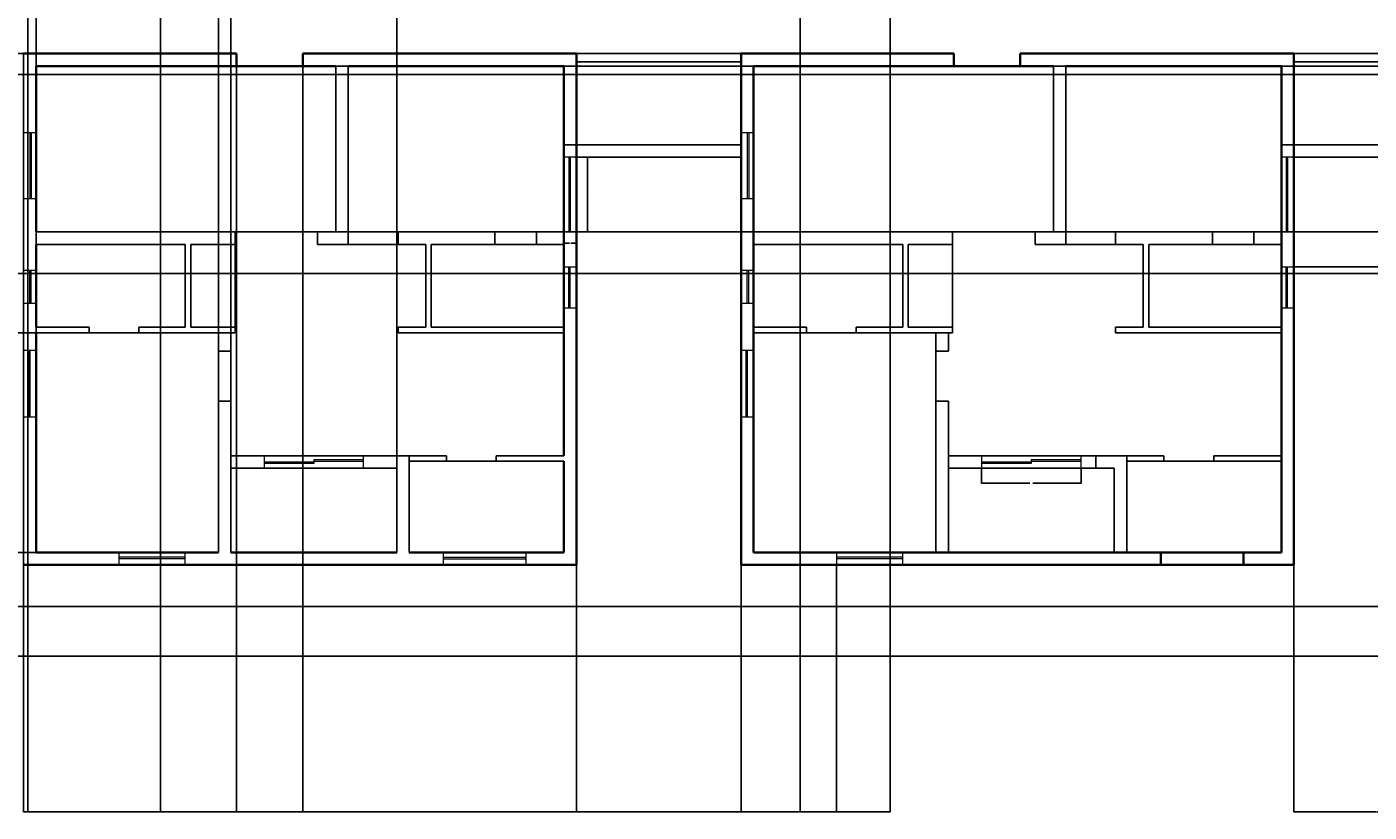
# Model space of a CAD drawing. Units: inches. Extents: x 2029 to 8798, y 1998 to 6373.
# Tile 4 of 11: x 2855 to 3826, y 4031 to 4599. Entities that reach past the tile are written whole.
import ezdxf

# ---------------------------------------------------------------- set-up
doc = ezdxf.new("R2010")
doc.units = ezdxf.units.IN
for name, color, linetype, lineweight in [('A-ANNO-DIMS', 2, 'Continuous', 18), ('A-GLAZ', 4, 'Continuous', 18), ('A-WALL-CIRC', 7, 'Continuous', 25), ('A-WALL-EXTR', 7, 'Continuous', 35), ('A-WALL-INTR', 7, 'Continuous', 25)]:
    doc.layers.add(name, color=color, linetype=linetype, lineweight=lineweight)
doc.styles.get("Standard").update_dxf_attribs({"font": 'arial.ttf'})
doc.dimstyles.get("Standard").update_dxf_attribs({"dimtxt": 0.18, "dimasz": 0.18, "dimexe": 0.18, "dimexo": 0.0625, "dimgap": 0.09, "dimtad": 0, "dimtih": 1, "dimtoh": 1, "dimdec": 4, "dimzin": 0, "dimdsep": 46, "dimtxsty": 'Standard', "dimcen": 0.09, "dimadec": 0, "dimazin": 0, "dimtfac": 1, "dimtdec": 4, "dimtofl": 0, "dimtmove": 0, "dimatfit": 3, "dimfxl": 1, "dimtolj": 1, "dimtzin": 0, "dimarcsym": 0})

# ---------------------------------------------------------------- blocks, each defined once
blk = doc.blocks.new('WIN-60')
for p, q in [((0, 0), (0, 9)), ((0, 4.5), (60, 4.5)), ((0, 3.5), (60, 3.5)), ((60, 9), (60, 0))]:
    blk.add_line(p, q)
blk = doc.blocks.new('WIN-48')
for p, q in [((0, 48), (9, 48)), ((4.5, 48), (4.5, 0)), ((5.5, 48), (5.5, 0)), ((9, 0), (0, 0))]:
    blk.add_line(p, q)
blk = doc.blocks.new('WIN-30')
for p, q in [((0, 0), (0, 9)), ((0, 5.5), (30, 5.5)), ((0, 4.5), (30, 4.5)), ((30, 9), (30, 0))]:
    blk.add_line(p, q)
blk = doc.blocks.new('WIN-24')
for p, q in [((0, 0), (0, 9)), ((0, 4.5), (24, 4.5)), ((0, 3.5), (24, 3.5)), ((24, 9), (24, 0))]:
    blk.add_line(p, q)
blk = doc.blocks.new('GLAZ-SLIDER-72-H')
for p, q in [((0, 9), (0, 0)), ((0, 4.5), (36, 4.5)), ((36, 3.5), (0, 3.5)), ((72, 6), (36, 6)), ((36, 6), (36, 5)), ((36, 5), (72, 5)), ((36, 4.5), (36, 3.5)), ((36, 4.5), (36, 4.5)), ((72, 0), (72, 9)), ((72, 5), (72, 6))]:
    blk.add_line(p, q)
blk = doc.blocks.new('WIN-54')
for p, q in [((9, 54), (0, 54)), ((3.5, 54), (3.5, 0)), ((4.5, 54), (4.5, 0)), ((0, 0), (9, 0))]:
    blk.add_line(p, q)
blk = doc.blocks.new('*D29')
at = {"layer": 'A-ANNO-DIMS', "color": 0, "lineweight": -2, "transparency": 16777216}
for p, q in [((3545.77, 4279.93), (3545.77, 4269.01)), ((3617.77, 4279.93), (3617.77, 4269.01)), ((3545.95, 4269.19), (3580.75, 4269.19)), ((3617.59, 4269.19), (3582.78, 4269.19))]:
    blk.add_line(p, q, dxfattribs=at)
at = {"layer": 'A-ANNO-DIMS', "color": 0, "transparency": 16777216}
for points in [[(3545.95, 4269.22), (3545.95, 4269.16), (3545.77, 4269.19)], [(3617.59, 4269.22), (3617.59, 4269.16), (3617.77, 4269.19)]]:
    blk.add_solid(points, dxfattribs=at)
at = {"layer": 'Defpoints', "color": 0, "transparency": 16777216}
for p in [(3545.77, 4279.99), (3617.77, 4279.99), (3617.77, 4269.19)]:
    blk.add_point(p, dxfattribs=at)
at = {"layer": 'A-ANNO-DIMS', "color": 0, "transparency": 16777216, "insert": (3581.77, 4269.19), "char_height": 0.18, "attachment_point": 5}
blk.add_mtext('\\A1;SLIDER 72 TYP.', dxfattribs=at)
blk = doc.blocks.new('*D30')
at = {"layer": 'A-ANNO-DIMS', "color": 0, "lineweight": -2, "transparency": 16777216}
for p, q in [((3617.83, 4288.99), (3628.75, 4288.99)), ((3628.57, 4288.81), (3628.57, 4284.67)), ((3628.57, 4280.17), (3628.57, 4284.31)), ((3617.83, 4279.99), (3628.75, 4279.99))]:
    blk.add_line(p, q, dxfattribs=at)
at = {"layer": 'A-ANNO-DIMS', "color": 0, "transparency": 16777216}
for points in [[(3628.54, 4288.81), (3628.6, 4288.81), (3628.57, 4288.99)], [(3628.54, 4280.17), (3628.6, 4280.17), (3628.57, 4279.99)]]:
    blk.add_solid(points, dxfattribs=at)
at = {"layer": 'Defpoints', "color": 0, "transparency": 16777216}
for p in [(3617.77, 4288.99), (3628.57, 4288.99), (3617.77, 4279.99)]:
    blk.add_point(p, dxfattribs=at)
at = {"layer": 'A-ANNO-DIMS', "color": 0, "transparency": 16777216, "insert": (3628.57, 4284.49), "char_height": 0.18, "attachment_point": 5}
blk.add_mtext('\\A1;9 TYP.', dxfattribs=at)
blk = doc.blocks.new('*D31')
at = {"layer": 'A-ANNO-DIMS', "color": 0, "lineweight": -2, "transparency": 16777216}
for p, q in [((3252.6, 4504.99), (3260.82, 4504.99)), ((3260.64, 4504.81), (3260.64, 4478.17)), ((3260.64, 4451.17), (3260.64, 4477.81)), ((3252.6, 4450.99), (3260.82, 4450.99))]:
    blk.add_line(p, q, dxfattribs=at)
at = {"layer": 'A-ANNO-DIMS', "color": 0, "transparency": 16777216}
for points in [[(3260.61, 4504.81), (3260.67, 4504.81), (3260.64, 4504.99)], [(3260.61, 4451.17), (3260.67, 4451.17), (3260.64, 4450.99)]]:
    blk.add_solid(points, dxfattribs=at)
at = {"layer": 'Defpoints', "color": 0, "transparency": 16777216}
for p in [(3252.54, 4504.99), (3260.64, 4504.99), (3252.54, 4450.99)]:
    blk.add_point(p, dxfattribs=at)
at = {"layer": 'A-ANNO-DIMS', "color": 0, "transparency": 16777216, "insert": (3260.64, 4477.99), "char_height": 0.18, "attachment_point": 5}
blk.add_mtext('\\A1;WINDOW 54 TYP.', dxfattribs=at)
blk = doc.blocks.new('*D32')
at = {"layer": 'A-ANNO-DIMS', "color": 0, "lineweight": -2, "transparency": 16777216}
for p, q in [((3243.54, 4450.93), (3243.54, 4442.71)), ((3252.54, 4450.93), (3252.54, 4442.71)), ((3243.72, 4442.89), (3247.58, 4442.89)), ((3252.36, 4442.89), (3248.5, 4442.89))]:
    blk.add_line(p, q, dxfattribs=at)
at = {"layer": 'A-ANNO-DIMS', "color": 0, "transparency": 16777216}
for points in [[(3243.72, 4442.92), (3243.72, 4442.86), (3243.54, 4442.89)], [(3252.36, 4442.92), (3252.36, 4442.86), (3252.54, 4442.89)]]:
    blk.add_solid(points, dxfattribs=at)
at = {"layer": 'Defpoints', "color": 0, "transparency": 16777216}
for p in [(3243.54, 4450.99), (3252.54, 4450.99), (3252.54, 4442.89)]:
    blk.add_point(p, dxfattribs=at)
at = {"layer": 'A-ANNO-DIMS', "color": 0, "transparency": 16777216, "insert": (3248.04, 4442.89), "char_height": 0.18, "attachment_point": 5}
blk.add_mtext('\\A1;9 TYP.', dxfattribs=at)
blk = doc.blocks.new('*D39')
at = {"layer": 'A-ANNO-DIMS', "color": 0, "lineweight": -2, "transparency": 16777216}
for p, q in [((2852.54, 4209.93), (2852.54, 4031.06)), ((3252.54, 4209.93), (3252.54, 4031.06)), ((2852.72, 4031.24), (3052.25, 4031.24)), ((3252.36, 4031.24), (3052.83, 4031.24))]:
    blk.add_line(p, q, dxfattribs=at)
at = {"layer": 'A-ANNO-DIMS', "color": 0, "transparency": 16777216}
for points in [[(2852.72, 4031.27), (2852.72, 4031.21), (2852.54, 4031.24)], [(3252.36, 4031.27), (3252.36, 4031.21), (3252.54, 4031.24)]]:
    blk.add_solid(points, dxfattribs=at)
at = {"layer": 'Defpoints', "color": 0, "transparency": 16777216}
for p in [(2852.54, 4209.99), (3252.54, 4209.99), (3252.54, 4031.24)]:
    blk.add_point(p, dxfattribs=at)
at = {"layer": 'A-ANNO-DIMS', "color": 0, "transparency": 16777216, "insert": (3052.54, 4031.24), "char_height": 0.18, "attachment_point": 5}
blk.add_mtext('\\A1;400', dxfattribs=at)
blk = doc.blocks.new('*D40')
at = {"layer": 'A-ANNO-DIMS', "color": 0, "lineweight": -2, "transparency": 16777216}
for p, q in [((3252.54, 4209.93), (3252.54, 4031.06)), ((3371.77, 4209.93), (3371.77, 4031.06)), ((3252.72, 4031.24), (3311.7, 4031.24)), ((3371.59, 4031.24), (3312.61, 4031.24))]:
    blk.add_line(p, q, dxfattribs=at)
at = {"layer": 'A-ANNO-DIMS', "color": 0, "transparency": 16777216}
for points in [[(3252.72, 4031.27), (3252.72, 4031.21), (3252.54, 4031.24)], [(3371.59, 4031.27), (3371.59, 4031.21), (3371.77, 4031.24)]]:
    blk.add_solid(points, dxfattribs=at)
at = {"layer": 'Defpoints', "color": 0, "transparency": 16777216}
for p in [(3252.54, 4209.99), (3371.77, 4209.99), (3371.77, 4031.24)]:
    blk.add_point(p, dxfattribs=at)
at = {"layer": 'A-ANNO-DIMS', "color": 0, "transparency": 16777216, "insert": (3312.15, 4031.24), "char_height": 0.18, "attachment_point": 5}
blk.add_mtext('\\A1;119.23', dxfattribs=at)
blk = doc.blocks.new('*D41')
at = {"layer": 'A-ANNO-DIMS', "color": 0, "lineweight": -2, "transparency": 16777216}
for p, q in [((3771.77, 4209.93), (3771.77, 4031.06)), ((3890.77, 4179.93), (3890.77, 4031.06)), ((3771.95, 4031.24), (3830.99, 4031.24)), ((3890.59, 4031.24), (3831.55, 4031.24))]:
    blk.add_line(p, q, dxfattribs=at)
at = {"layer": 'A-ANNO-DIMS', "color": 0, "transparency": 16777216}
for points in [[(3771.95, 4031.27), (3771.95, 4031.21), (3771.77, 4031.24)], [(3890.59, 4031.27), (3890.59, 4031.21), (3890.77, 4031.24)]]:
    blk.add_solid(points, dxfattribs=at)
at = {"layer": 'Defpoints', "color": 0, "transparency": 16777216}
for p in [(3771.77, 4209.99), (3890.77, 4179.99), (3890.77, 4031.24)]:
    blk.add_point(p, dxfattribs=at)
at = {"layer": 'A-ANNO-DIMS', "color": 0, "transparency": 16777216, "insert": (3831.27, 4031.24), "char_height": 0.18, "attachment_point": 5}
blk.add_mtext('\\A1;119', dxfattribs=at)
blk = doc.blocks.new('*D50')
at = {"layer": 'A-ANNO-DIMS', "color": 0, "lineweight": -2, "transparency": 16777216}
for p, q in [((2852.54, 4579.93), (2852.54, 4031.06)), ((3006.54, 4579.93), (3006.54, 4031.06)), ((2852.72, 4031.24), (2929.26, 4031.24)), ((3006.36, 4031.24), (2929.82, 4031.24))]:
    blk.add_line(p, q, dxfattribs=at)
at = {"layer": 'A-ANNO-DIMS', "color": 0, "transparency": 16777216}
for points in [[(2852.72, 4031.27), (2852.72, 4031.21), (2852.54, 4031.24)], [(3006.36, 4031.27), (3006.36, 4031.21), (3006.54, 4031.24)]]:
    blk.add_solid(points, dxfattribs=at)
at = {"layer": 'Defpoints', "color": 0, "transparency": 16777216}
for p in [(2852.54, 4579.99), (3006.54, 4579.99), (3006.54, 4031.24)]:
    blk.add_point(p, dxfattribs=at)
at = {"layer": 'A-ANNO-DIMS', "color": 0, "transparency": 16777216, "insert": (2929.54, 4031.24), "char_height": 0.18, "attachment_point": 5}
blk.add_mtext('\\A1;154', dxfattribs=at)
blk = doc.blocks.new('*D51')
at = {"layer": 'A-ANNO-DIMS', "color": 0, "lineweight": -2, "transparency": 16777216}
for p, q in [((3006.54, 4579.93), (3006.54, 4031.06)), ((3054.54, 4579.93), (3054.54, 4031.06)), ((3006.72, 4031.24), (3030.32, 4031.24)), ((3054.36, 4031.24), (3030.76, 4031.24))]:
    blk.add_line(p, q, dxfattribs=at)
at = {"layer": 'A-ANNO-DIMS', "color": 0, "transparency": 16777216}
for points in [[(3006.72, 4031.27), (3006.72, 4031.21), (3006.54, 4031.24)], [(3054.36, 4031.27), (3054.36, 4031.21), (3054.54, 4031.24)]]:
    blk.add_solid(points, dxfattribs=at)
at = {"layer": 'Defpoints', "color": 0, "transparency": 16777216}
for p in [(3006.54, 4579.99), (3054.54, 4579.99), (3054.54, 4031.24)]:
    blk.add_point(p, dxfattribs=at)
at = {"layer": 'A-ANNO-DIMS', "color": 0, "transparency": 16777216, "insert": (3030.54, 4031.24), "char_height": 0.18, "attachment_point": 5}
blk.add_mtext('\\A1;48', dxfattribs=at)
blk = doc.blocks.new('*D52')
at = {"layer": 'A-ANNO-DIMS', "color": 0, "lineweight": -2, "transparency": 16777216}
for p, q in [((2861.6, 4570.99), (4503.7, 4570.99)), ((4503.52, 4570.81), (4503.52, 4511.17)), ((4503.52, 4451.17), (4503.52, 4510.81)), ((2861.6, 4450.99), (4503.7, 4450.99))]:
    blk.add_line(p, q, dxfattribs=at)
at = {"layer": 'A-ANNO-DIMS', "color": 0, "transparency": 16777216}
for points in [[(4503.49, 4570.81), (4503.55, 4570.81), (4503.52, 4570.99)], [(4503.49, 4451.17), (4503.55, 4451.17), (4503.52, 4450.99)]]:
    blk.add_solid(points, dxfattribs=at)
at = {"layer": 'Defpoints', "color": 0, "transparency": 16777216}
for p in [(2861.54, 4570.99), (4503.52, 4570.99), (2861.54, 4450.99)]:
    blk.add_point(p, dxfattribs=at)
at = {"layer": 'A-ANNO-DIMS', "color": 0, "transparency": 16777216, "insert": (4503.52, 4510.99), "char_height": 0.18, "attachment_point": 5}
blk.add_mtext('\\A1;120', dxfattribs=at)
blk = doc.blocks.new('*D53')
at = {"layer": 'A-ANNO-DIMS', "color": 0, "lineweight": -2, "transparency": 16777216}
for p, q in [((2861.48, 4377.99), (2029.61, 4377.99)), ((2029.79, 4377.81), (2029.79, 4298.67)), ((2029.79, 4219.17), (2029.79, 4298.31)), ((2861.48, 4218.99), (2029.61, 4218.99))]:
    blk.add_line(p, q, dxfattribs=at)
at = {"layer": 'A-ANNO-DIMS', "color": 0, "transparency": 16777216}
for points in [[(2029.76, 4377.81), (2029.82, 4377.81), (2029.79, 4377.99)], [(2029.76, 4219.17), (2029.82, 4219.17), (2029.79, 4218.99)]]:
    blk.add_solid(points, dxfattribs=at)
at = {"layer": 'Defpoints', "color": 0, "transparency": 16777216}
for p in [(2861.54, 4377.99), (2029.79, 4218.99), (2861.54, 4218.99)]:
    blk.add_point(p, dxfattribs=at)
at = {"layer": 'A-ANNO-DIMS', "color": 0, "transparency": 16777216, "insert": (2029.79, 4298.49), "char_height": 0.18, "attachment_point": 5}
blk.add_mtext('\\A1;159', dxfattribs=at)
blk = doc.blocks.new('*D54')
at = {"layer": 'A-ANNO-DIMS', "color": 0, "lineweight": -2, "transparency": 16777216}
for p, q in [((2861.54, 4219.05), (2861.54, 6372.54)), ((2861.72, 6372.36), (2927.26, 6372.36)), ((2993.36, 6372.36), (2927.82, 6372.36)), ((2993.54, 4219.05), (2993.54, 6372.54))]:
    blk.add_line(p, q, dxfattribs=at)
at = {"layer": 'A-ANNO-DIMS', "color": 0, "transparency": 16777216}
for points in [[(2861.72, 6372.39), (2861.72, 6372.33), (2861.54, 6372.36)], [(2993.36, 6372.39), (2993.36, 6372.33), (2993.54, 6372.36)]]:
    blk.add_solid(points, dxfattribs=at)
at = {"layer": 'Defpoints', "color": 0, "transparency": 16777216}
for p in [(2993.54, 6372.36), (2861.54, 4218.99), (2993.54, 4218.99)]:
    blk.add_point(p, dxfattribs=at)
at = {"layer": 'A-ANNO-DIMS', "color": 0, "transparency": 16777216, "insert": (2927.54, 6372.36), "char_height": 0.18, "attachment_point": 5}
blk.add_mtext('\\A1;132', dxfattribs=at)
blk = doc.blocks.new('*D55')
at = {"layer": 'A-ANNO-DIMS', "color": 0, "lineweight": -2, "transparency": 16777216}
for p, q in [((3002.54, 4219.05), (3002.54, 6372.54)), ((3002.72, 6372.36), (3062.26, 6372.36)), ((3122.36, 6372.36), (3062.82, 6372.36)), ((3122.54, 4219.05), (3122.54, 6372.54))]:
    blk.add_line(p, q, dxfattribs=at)
at = {"layer": 'A-ANNO-DIMS', "color": 0, "transparency": 16777216}
for points in [[(3002.72, 6372.39), (3002.72, 6372.33), (3002.54, 6372.36)], [(3122.36, 6372.39), (3122.36, 6372.33), (3122.54, 6372.36)]]:
    blk.add_solid(points, dxfattribs=at)
at = {"layer": 'Defpoints', "color": 0, "transparency": 16777216}
for p in [(3122.54, 6372.36), (3002.54, 4218.99), (3122.54, 4218.99)]:
    blk.add_point(p, dxfattribs=at)
at = {"layer": 'A-ANNO-DIMS', "color": 0, "transparency": 16777216, "insert": (3062.54, 6372.36), "char_height": 0.18, "attachment_point": 5}
blk.add_mtext('\\A1;120', dxfattribs=at)
blk = doc.blocks.new('*D56')
at = {"layer": 'A-ANNO-DIMS', "color": 0, "lineweight": -2, "transparency": 16777216}
for p, q in [((3371.77, 4209.93), (3371.77, 4031.06)), ((3440.77, 4209.93), (3440.77, 4031.06)), ((3371.95, 4031.24), (3406.05, 4031.24)), ((3440.59, 4031.24), (3406.49, 4031.24))]:
    blk.add_line(p, q, dxfattribs=at)
at = {"layer": 'A-ANNO-DIMS', "color": 0, "transparency": 16777216}
for points in [[(3371.95, 4031.27), (3371.95, 4031.21), (3371.77, 4031.24)], [(3440.59, 4031.27), (3440.59, 4031.21), (3440.77, 4031.24)]]:
    blk.add_solid(points, dxfattribs=at)
at = {"layer": 'Defpoints', "color": 0, "transparency": 16777216}
for p in [(3371.77, 4209.99), (3440.77, 4209.99), (3440.77, 4031.24)]:
    blk.add_point(p, dxfattribs=at)
at = {"layer": 'A-ANNO-DIMS', "color": 0, "transparency": 16777216, "insert": (3406.27, 4031.24), "char_height": 0.18, "attachment_point": 5}
blk.add_mtext('\\A1;69', dxfattribs=at)
blk = doc.blocks.new('*D57')
at = {"layer": 'A-ANNO-DIMS', "color": 0, "lineweight": -2, "transparency": 16777216}
for p, q in [((3771.83, 4579.99), (4503.7, 4579.99)), ((4503.52, 4579.81), (4503.52, 4542.67)), ((4503.52, 4505.17), (4503.52, 4542.31)), ((3771.83, 4504.99), (4503.7, 4504.99))]:
    blk.add_line(p, q, dxfattribs=at)
at = {"layer": 'A-ANNO-DIMS', "color": 0, "transparency": 16777216}
for points in [[(4503.49, 4579.81), (4503.55, 4579.81), (4503.52, 4579.99)], [(4503.49, 4505.17), (4503.55, 4505.17), (4503.52, 4504.99)]]:
    blk.add_solid(points, dxfattribs=at)
at = {"layer": 'Defpoints', "color": 0, "transparency": 16777216}
for p in [(3771.77, 4579.99), (3771.77, 4504.99), (4503.52, 4504.99)]:
    blk.add_point(p, dxfattribs=at)
at = {"layer": 'A-ANNO-DIMS', "color": 0, "transparency": 16777216, "insert": (4503.52, 4542.49), "char_height": 0.18, "attachment_point": 5}
blk.add_mtext('\\A1;75', dxfattribs=at)
blk = doc.blocks.new('*D58')
at = {"layer": 'A-ANNO-DIMS', "color": 0, "lineweight": -2, "transparency": 16777216}
for p, q in [((3771.83, 4450.99), (4503.7, 4450.99)), ((4503.52, 4450.81), (4503.52, 4438.52)), ((4503.52, 4425.88), (4503.52, 4438.16)), ((3771.83, 4425.7), (4503.7, 4425.7))]:
    blk.add_line(p, q, dxfattribs=at)
at = {"layer": 'A-ANNO-DIMS', "color": 0, "transparency": 16777216}
for points in [[(4503.49, 4450.81), (4503.55, 4450.81), (4503.52, 4450.99)], [(4503.49, 4425.88), (4503.55, 4425.88), (4503.52, 4425.7)]]:
    blk.add_solid(points, dxfattribs=at)
at = {"layer": 'Defpoints', "color": 0, "transparency": 16777216}
for p in [(3771.77, 4450.99), (3771.77, 4425.7), (4503.52, 4425.7)]:
    blk.add_point(p, dxfattribs=at)
at = {"layer": 'A-ANNO-DIMS', "color": 0, "transparency": 16777216, "insert": (4503.52, 4438.34), "char_height": 0.18, "attachment_point": 5}
blk.add_mtext('\\A1;25.293', dxfattribs=at)
blk = doc.blocks.new('*D59')
at = {"layer": 'A-ANNO-DIMS', "color": 0, "lineweight": -2, "transparency": 16777216}
for p, q in [((2951.53, 4953.93), (2951.53, 4031.06)), ((3414.53, 4953.93), (3414.53, 4031.06)), ((2951.71, 4031.24), (3182.74, 4031.24)), ((3414.35, 4031.24), (3183.32, 4031.24))]:
    blk.add_line(p, q, dxfattribs=at)
at = {"layer": 'A-ANNO-DIMS', "color": 0, "transparency": 16777216}
for points in [[(2951.71, 4031.27), (2951.71, 4031.21), (2951.53, 4031.24)], [(3414.35, 4031.27), (3414.35, 4031.21), (3414.53, 4031.24)]]:
    blk.add_solid(points, dxfattribs=at)
at = {"layer": 'Defpoints', "color": 0, "transparency": 16777216}
for p in [(2951.53, 4953.99), (3414.53, 4953.99), (3414.53, 4031.24)]:
    blk.add_point(p, dxfattribs=at)
at = {"layer": 'A-ANNO-DIMS', "color": 0, "transparency": 16777216, "insert": (3183.03, 4031.24), "char_height": 0.18, "attachment_point": 5}
blk.add_mtext('\\A1;463', dxfattribs=at)
blk = doc.blocks.new('*D67')
at = {"layer": 'A-ANNO-DIMS', "color": 0, "lineweight": -2, "transparency": 16777216}
for p, q in [((2855.53, 4657.93), (2855.53, 4031.06)), ((3479.53, 4657.93), (3479.53, 4031.06)), ((2855.71, 4031.24), (3167.24, 4031.24)), ((3479.35, 4031.24), (3167.82, 4031.24))]:
    blk.add_line(p, q, dxfattribs=at)
at = {"layer": 'A-ANNO-DIMS', "color": 0, "transparency": 16777216}
for points in [[(2855.71, 4031.27), (2855.71, 4031.21), (2855.53, 4031.24)], [(3479.35, 4031.27), (3479.35, 4031.21), (3479.53, 4031.24)]]:
    blk.add_solid(points, dxfattribs=at)
at = {"layer": 'Defpoints', "color": 0, "transparency": 16777216}
for p in [(2855.53, 4657.99), (3479.53, 4657.99), (3479.53, 4031.24)]:
    blk.add_point(p, dxfattribs=at)
at = {"layer": 'A-ANNO-DIMS', "color": 0, "transparency": 16777216, "insert": (3167.53, 4031.24), "char_height": 0.18, "attachment_point": 5}
blk.add_mtext('\\A1;624', dxfattribs=at)
blk = doc.blocks.new('*D86')
at = {"layer": 'A-ANNO-DIMS', "color": 0, "lineweight": -2, "transparency": 16777216}
for p, q in [((4373.7, 4564.99), (2029.61, 4564.99)), ((2029.79, 4564.81), (2029.79, 4493.17)), ((2029.79, 4421.17), (2029.79, 4492.81)), ((4373.7, 4420.99), (2029.61, 4420.99))]:
    blk.add_line(p, q, dxfattribs=at)
at = {"layer": 'A-ANNO-DIMS', "color": 0, "transparency": 16777216}
for points in [[(2029.76, 4564.81), (2029.82, 4564.81), (2029.79, 4564.99)], [(2029.76, 4421.17), (2029.82, 4421.17), (2029.79, 4420.99)]]:
    blk.add_solid(points, dxfattribs=at)
at = {"layer": 'Defpoints', "color": 0, "transparency": 16777216}
for p in [(4373.77, 4564.99), (2029.79, 4420.99), (4373.77, 4420.99)]:
    blk.add_point(p, dxfattribs=at)
at = {"layer": 'A-ANNO-DIMS', "color": 0, "transparency": 16777216, "insert": (2029.79, 4492.99), "char_height": 0.18, "attachment_point": 5}
blk.add_mtext('\\A1;144', dxfattribs=at)
blk = doc.blocks.new('*D88')
at = {"layer": 'A-ANNO-DIMS', "color": 0, "lineweight": -2, "transparency": 16777216}
for p, q in [((2142.54, 4445.05), (2142.54, 6372.54)), ((2142.72, 6372.36), (3266.19, 6372.36)), ((4390.59, 6372.36), (3267.12, 6372.36)), ((4390.77, 4574.05), (4390.77, 6372.54))]:
    blk.add_line(p, q, dxfattribs=at)
at = {"layer": 'A-ANNO-DIMS', "color": 0, "transparency": 16777216}
for points in [[(2142.72, 6372.39), (2142.72, 6372.33), (2142.54, 6372.36)], [(4390.59, 6372.39), (4390.59, 6372.33), (4390.77, 6372.36)]]:
    blk.add_solid(points, dxfattribs=at)
at = {"layer": 'Defpoints', "color": 0, "transparency": 16777216}
for p in [(4390.77, 6372.36), (4390.77, 4573.99), (2142.54, 4444.99)]:
    blk.add_point(p, dxfattribs=at)
at = {"layer": 'A-ANNO-DIMS', "color": 0, "transparency": 16777216, "insert": (3266.65, 6372.36), "char_height": 0.18, "attachment_point": 5}
blk.add_mtext('\\A1;2248.2', dxfattribs=at)
blk = doc.blocks.new('*D117')
at = {"layer": 'A-ANNO-DIMS', "color": 0, "lineweight": -2, "transparency": 16777216}
for p, q in [((4105.7, 4179.99), (2029.61, 4179.99)), ((2029.79, 4179.81), (2029.79, 4162.17)), ((2029.79, 4144.17), (2029.79, 4161.81)), ((4105.7, 4143.99), (2029.61, 4143.99))]:
    blk.add_line(p, q, dxfattribs=at)
at = {"layer": 'A-ANNO-DIMS', "color": 0, "transparency": 16777216}
for points in [[(2029.76, 4179.81), (2029.82, 4179.81), (2029.79, 4179.99)], [(2029.76, 4144.17), (2029.82, 4144.17), (2029.79, 4143.99)]]:
    blk.add_solid(points, dxfattribs=at)
at = {"layer": 'Defpoints', "color": 0, "transparency": 16777216}
for p in [(2029.79, 4179.99), (4105.77, 4179.99), (4105.77, 4143.99)]:
    blk.add_point(p, dxfattribs=at)
at = {"layer": 'A-ANNO-DIMS', "color": 0, "transparency": 16777216, "insert": (2029.79, 4161.99), "char_height": 0.18, "attachment_point": 5}
blk.add_mtext('\\A1;36', dxfattribs=at)

msp = doc.modelspace()

# ---------------------------------------------------------------- linework, layer by layer
at = {"layer": 'A-GLAZ'}
for p, q in [((3371.7657, 4474.9886), (3371.7657, 4522.9886)), ((3252.5398, 4425.6956), (3252.5398, 4395.6956)), ((3371.7657, 4399.2558), (3371.7657, 4423.2558)), ((3771.7657, 4425.6956), (3771.7657, 4395.6956)), ((3371.7657, 4365.0621), (3371.7657, 4317.0621)), ((2969.5398, 4209.9886), (2921.5398, 4209.9886)), ((3216.1929, 4209.9886), (3156.1929, 4209.9886)), ((3488.7657, 4209.9886), (3440.7657, 4209.9886))]:
    msp.add_line(p, q, dxfattribs=at)
at = {"layer": 'A-WALL-CIRC'}
for p, q in [((3006.5398, 4579.9886), (2417.7365, 4579.9886)), ((3371.7657, 4579.9886), (3054.5398, 4579.9886)), ((3371.5398, 4573.9886), (3252.5398, 4573.9886)), ((3890.7657, 4573.9886), (3771.7657, 4573.9886)), ((3243.5398, 4513.9886), (3371.5398, 4513.9886)), ((3762.7657, 4513.9886), (3890.7657, 4513.9886)), ((3371.5398, 4504.9886), (3251.5398, 4504.9886)), ((3890.7657, 4504.9886), (3770.7657, 4504.9886))]:
    msp.add_line(p, q, dxfattribs=at)
at = {"layer": 'A-WALL-EXTR'}
for p, q in [((2852.5398, 4579.9886), (2861.5398, 4579.9886)), ((3006.5398, 4579.9886), (2861.5398, 4579.9886)), ((3006.5398, 4579.9886), (3006.5398, 4570.9886)), ((3077.5398, 4579.9886), (3054.5398, 4579.9886)), ((3054.5398, 4570.9886), (3054.5398, 4579.9886)), ((3086.5398, 4579.9886), (3077.5398, 4579.9886)), ((3242.5398, 4579.9886), (3086.5398, 4579.9886)), ((3251.5398, 4579.9886), (3242.5398, 4579.9886)), ((3243.5398, 4579.9886), (3251.5398, 4579.9886)), ((3243.5398, 4579.9886), (3252.5398, 4579.9886)), ((3252.5398, 4579.9886), (3252.5398, 4209.9886)), ((3380.7657, 4579.9886), (3371.7657, 4579.9886)), ((3371.7657, 4579.9886), (3371.7657, 4570.9886)), ((3371.7657, 4579.9886), (3380.7657, 4579.9886)), ((3525.7657, 4579.9886), (3380.7657, 4579.9886)), ((3525.7657, 4579.9886), (3525.7657, 4570.9886)), ((3596.7657, 4579.9886), (3573.7657, 4579.9886)), ((3573.7657, 4570.9886), (3573.7657, 4579.9886)), ((3605.7657, 4579.9886), (3596.7657, 4579.9886)), ((3761.7657, 4579.9886), (3605.7657, 4579.9886)), ((3770.7657, 4579.9886), (3761.7657, 4579.9886)), ((3762.7657, 4579.9886), (3770.7657, 4579.9886)), ((3762.7657, 4579.9886), (3771.7657, 4579.9886)), ((3771.7657, 4579.9886), (3771.7657, 4209.9886)), ((3078.5398, 4570.9886), (2861.5398, 4570.9886)), ((2861.5398, 4570.9886), (2861.5398, 4450.9886)), ((2861.5398, 4570.9886), (2861.5398, 4450.9886)), ((3078.5398, 4570.9886), (3054.5398, 4570.9886)), ((3243.5398, 4570.9886), (3087.5398, 4570.9886)), ((3243.5398, 4570.9886), (3087.5398, 4570.9886)), ((3243.5398, 4570.9886), (3243.5398, 4450.9886)), ((3243.5398, 4288.9886), (3243.5398, 4570.9886)), ((3371.7657, 4570.9886), (3371.7657, 4450.9886)), ((3380.7657, 4570.9886), (3380.7657, 4218.9886)), ((3380.7657, 4570.9886), (3380.7657, 4450.9886)), ((3597.7657, 4570.9886), (3380.7657, 4570.9886)), ((3597.7657, 4570.9886), (3573.7657, 4570.9886)), ((3762.7657, 4570.9886), (3606.7657, 4570.9886)), ((3762.7657, 4570.9886), (3606.7657, 4570.9886)), ((3762.7657, 4218.9886), (3762.7657, 4570.9886)), ((3762.7657, 4570.9886), (3762.7657, 4450.9886)), ((3243.5398, 4504.9886), (3243.5398, 4513.9886)), ((3762.7657, 4504.9886), (3762.7657, 4513.9886)), ((2861.5398, 4450.9886), (2861.5398, 4474.9886)), ((3380.7657, 4450.9886), (3380.7657, 4474.9886)), ((3371.7657, 4450.9886), (3371.7657, 4441.9886)), ((2861.5398, 4441.9886), (2861.5398, 4381.9886)), ((2861.5398, 4441.9886), (2861.5398, 4381.9886)), ((3243.5398, 4441.9886), (3243.5398, 4381.9886)), ((3243.5398, 4441.9886), (3243.5398, 4425.6956)), ((3371.7657, 4441.9886), (3371.7657, 4381.9886)), ((3380.7657, 4441.9886), (3380.7657, 4381.9886)), ((3762.7657, 4441.9886), (3762.7657, 4381.9886)), ((3762.7657, 4441.9886), (3762.7657, 4425.6956)), ((2861.5398, 4381.9886), (2861.5398, 4399.2558)), ((3380.7657, 4381.9886), (3380.7657, 4399.2558)), ((3371.7657, 4381.9886), (3371.7657, 4377.9886)), ((2861.5398, 4377.9886), (2861.5398, 4365.0621)), ((2861.5398, 4377.9886), (2861.5398, 4218.9886)), ((3371.7657, 4377.9886), (3371.7657, 4218.9886)), ((3380.7657, 4377.9886), (3380.7657, 4365.0621)), ((3243.5398, 4218.9886), (3243.5398, 4284.9886)), ((3762.7657, 4288.9886), (3762.7657, 4284.9886)), ((2861.5398, 4218.9886), (2993.5398, 4218.9886)), ((2861.5398, 4218.9886), (2993.5398, 4218.9886)), ((2993.5398, 4218.9886), (2969.5398, 4218.9886)), ((3002.5398, 4218.9886), (3122.5398, 4218.9886)), ((3002.5398, 4218.9886), (3122.5398, 4218.9886)), ((3131.5588, 4218.9886), (3243.5398, 4218.9886)), ((3243.5398, 4218.9886), (3216.1929, 4218.9886)), ((3371.7657, 4218.9886), (3371.7657, 4209.9886)), ((3371.7657, 4209.9886), (3371.7657, 4218.9886)), ((3380.7657, 4218.9886), (3762.7657, 4218.9886)), ((3380.7657, 4218.9886), (3512.7657, 4218.9886)), ((3512.7657, 4218.9886), (3488.7657, 4218.9886)), ((3521.7657, 4218.9886), (3641.7657, 4218.9886)), ((3675.4188, 4209.9886), (3675.4188, 4218.9886)), ((3762.7657, 4218.9886), (3735.4188, 4218.9886)), ((3735.4188, 4218.9886), (3735.4188, 4209.9886)), ((2852.5398, 4209.9886), (2861.5398, 4209.9886)), ((2861.5398, 4209.9886), (2993.5398, 4209.9886)), ((2993.5398, 4209.9886), (3002.5398, 4209.9886)), ((3002.5398, 4209.9886), (3122.5398, 4209.9886)), ((3122.5398, 4209.9886), (3131.5398, 4209.9886)), ((3131.5398, 4209.9886), (3243.5398, 4209.9886)), ((3252.5398, 4209.9886), (3243.5398, 4209.9886)), ((3371.7657, 4209.9886), (3380.7657, 4209.9886)), ((3380.7657, 4209.9886), (3512.7657, 4209.9886)), ((3512.7657, 4209.9886), (3521.7657, 4209.9886)), ((3521.7657, 4209.9886), (3641.7657, 4209.9886)), ((3641.7657, 4209.9886), (3650.7657, 4209.9886)), ((3650.7657, 4209.9886), (3762.7657, 4209.9886)), ((3735.4188, 4209.9886), (3675.4188, 4209.9886)), ((3771.7657, 4209.9886), (3762.7657, 4209.9886))]:
    msp.add_line(p, q, dxfattribs=at)
at = {"layer": 'A-WALL-INTR'}
for p, q in [((3078.5398, 4450.9886), (3078.5398, 4570.9886)), ((3087.5398, 4570.9886), (3087.5398, 4450.9886)), ((3597.7657, 4450.9886), (3597.7657, 4570.9886)), ((3606.7657, 4570.9886), (3606.7657, 4450.9886)), ((2861.5398, 4450.9886), (3005.5398, 4450.9886)), ((3005.5398, 4441.9886), (3005.5398, 4450.9886)), ((3065.2881, 4450.9886), (3078.5398, 4450.9886)), ((3078.5398, 4450.9886), (3065.2881, 4450.9886)), ((3065.2881, 4450.9886), (3065.2881, 4441.9886)), ((3087.5398, 4450.9886), (3087.5398, 4441.9886)), ((3087.5398, 4450.9886), (3087.5398, 4441.9886)), ((3193.6, 4450.9886), (3123.5398, 4450.9886)), ((3123.5398, 4441.9886), (3123.5398, 4450.9886)), ((3193.6, 4441.9886), (3193.6, 4450.9886)), ((3243.5398, 4450.9886), (3223.6, 4450.9886)), ((3243.5398, 4450.9886), (3223.6, 4450.9886)), ((3223.6, 4450.9886), (3223.6, 4441.9886)), ((3380.7657, 4450.9886), (3524.7657, 4450.9886)), ((3524.7657, 4441.9886), (3524.7657, 4450.9886)), ((3597.7657, 4450.9886), (3584.514, 4450.9886)), ((3584.514, 4450.9886), (3584.514, 4441.9886)), ((3584.514, 4450.9886), (3597.7657, 4450.9886)), ((3606.7657, 4450.9886), (3606.7657, 4441.9886)), ((3606.7657, 4450.9886), (3606.7657, 4441.9886)), ((3642.7657, 4441.9886), (3642.7657, 4450.9886)), ((3712.8259, 4450.9886), (3642.7657, 4450.9886)), ((3712.8259, 4441.9886), (3712.8259, 4450.9886)), ((3762.7657, 4450.9886), (3742.8259, 4450.9886)), ((3762.7657, 4450.9886), (3742.8259, 4450.9886)), ((3742.8259, 4450.9886), (3742.8259, 4441.9886)), ((2969.5398, 4441.9886), (2861.5398, 4441.9886)), ((2969.5398, 4381.9886), (2969.5398, 4441.9886)), ((3005.5398, 4441.9886), (2973.5398, 4441.9886)), ((2973.5398, 4441.9886), (2973.5398, 4381.9886)), ((3005.5398, 4381.9886), (3005.5398, 4441.9886)), ((3087.5398, 4441.9886), (3065.2881, 4441.9886)), ((3087.5398, 4441.9886), (3143.5398, 4441.9886)), ((3087.5398, 4441.9886), (3123.5398, 4441.9886)), ((3143.5398, 4441.9886), (3143.5398, 4437.9886)), ((3147.5398, 4441.9886), (3243.5398, 4441.9886)), ((3147.5398, 4381.9886), (3147.5398, 4441.9886)), ((3223.6, 4441.9886), (3193.6, 4441.9886)), ((3488.7657, 4441.9886), (3380.7657, 4441.9886)), ((3488.7657, 4381.9886), (3488.7657, 4441.9886)), ((3492.7657, 4441.9886), (3492.7657, 4381.9886)), ((3524.7657, 4441.9886), (3492.7657, 4441.9886)), ((3524.7657, 4381.9886), (3524.7657, 4441.9886)), ((3606.7657, 4441.9886), (3584.514, 4441.9886)), ((3606.7657, 4441.9886), (3662.7657, 4441.9886)), ((3606.7657, 4441.9886), (3642.7657, 4441.9886)), ((3662.7657, 4441.9886), (3662.7657, 4437.9886)), ((3666.7657, 4381.9886), (3666.7657, 4441.9886)), ((3666.7657, 4441.9886), (3762.7657, 4441.9886)), ((3742.8259, 4441.9886), (3712.8259, 4441.9886)), ((3143.5398, 4437.9886), (3143.5398, 4381.9886)), ((3662.7657, 4437.9886), (3662.7657, 4381.9886)), ((2861.5398, 4381.9886), (2899.9258, 4381.9886)), ((2899.9258, 4377.9886), (2899.9258, 4381.9886)), ((2935.9258, 4381.9886), (2969.5398, 4381.9886)), ((2969.5398, 4381.9886), (2935.9258, 4381.9886)), ((2935.9258, 4381.9886), (2935.9258, 4377.9886)), ((2973.5398, 4381.9886), (3005.5398, 4381.9886)), ((3005.5398, 4381.9886), (3005.5398, 4377.9886)), ((3123.5398, 4377.9886), (3123.5398, 4381.9886)), ((3123.5398, 4381.9886), (3143.5398, 4381.9886)), ((3243.5398, 4381.9886), (3147.5398, 4381.9886)), ((3380.7657, 4381.9886), (3419.1517, 4381.9886)), ((3419.1517, 4377.9886), (3419.1517, 4381.9886)), ((3488.7657, 4381.9886), (3455.1517, 4381.9886)), ((3455.1517, 4381.9886), (3455.1517, 4377.9886)), ((3455.1517, 4381.9886), (3488.7657, 4381.9886)), ((3492.7657, 4381.9886), (3524.7657, 4381.9886)), ((3524.7657, 4381.9886), (3524.7657, 4377.9886)), ((3642.7657, 4377.9886), (3642.7657, 4381.9886)), ((3642.7657, 4381.9886), (3662.7657, 4381.9886)), ((3762.7657, 4381.9886), (3666.7657, 4381.9886)), ((2973.5398, 4377.9886), (2861.5398, 4377.9886)), ((2935.9258, 4377.9886), (2899.9258, 4377.9886)), ((3005.5398, 4377.9886), (2973.5398, 4377.9886)), ((2993.5398, 4218.9886), (2993.5398, 4377.9886)), ((2993.5398, 4377.9886), (3002.5398, 4377.9886)), ((3002.5398, 4377.9886), (3002.5398, 4364.5574)), ((3002.5398, 4377.9886), (3002.5398, 4364.5574)), ((3143.5398, 4377.9886), (3123.5398, 4377.9886)), ((3143.5398, 4377.9886), (3243.5398, 4377.9886)), ((3492.7657, 4377.9886), (3380.7657, 4377.9886)), ((3455.1517, 4377.9886), (3419.1517, 4377.9886)), ((3524.7657, 4377.9886), (3492.7657, 4377.9886)), ((3512.7657, 4218.9886), (3512.7657, 4377.9886)), ((3512.7657, 4377.9886), (3521.7657, 4377.9886)), ((3521.7657, 4377.9886), (3521.7657, 4364.5574)), ((3521.7657, 4377.9886), (3521.7657, 4364.5574)), ((3662.7657, 4377.9886), (3642.7657, 4377.9886)), ((3662.7657, 4377.9886), (3762.7657, 4377.9886)), ((3002.5398, 4364.5574), (2993.5398, 4364.5574)), ((2993.5398, 4364.5574), (2993.5398, 4328.5574)), ((3521.7657, 4364.5574), (3512.7657, 4364.5574)), ((3512.7657, 4364.5574), (3512.7657, 4328.5574)), ((2993.5398, 4328.5574), (3002.5398, 4328.5574)), ((3002.5398, 4328.5574), (3002.5398, 4288.9886)), ((3512.7657, 4328.5574), (3521.7657, 4328.5574)), ((3521.7657, 4328.5574), (3521.7657, 4218.9886)), ((3002.5398, 4288.9886), (3122.5588, 4288.9886)), ((3002.5398, 4288.9886), (3026.5398, 4288.9886)), ((3122.5588, 4288.9886), (3131.5588, 4288.9886)), ((3131.5588, 4288.9886), (3131.5588, 4218.9886)), ((3131.5588, 4288.9886), (3134.5588, 4288.9886)), ((3158.5588, 4284.9886), (3131.5588, 4284.9886)), ((3134.5588, 4288.9886), (3158.5588, 4288.9886)), ((3158.5588, 4288.9886), (3158.5588, 4284.9886)), ((3158.5588, 4284.9886), (3194.5588, 4284.9886)), ((3194.5588, 4284.9886), (3194.5588, 4288.9886)), ((3194.5588, 4288.9886), (3243.5398, 4288.9886)), ((3243.5398, 4284.9886), (3194.5588, 4284.9886)), ((3521.7657, 4279.9886), (3521.7657, 4288.9886)), ((3521.7657, 4288.9886), (3641.7847, 4288.9886)), ((3521.7657, 4288.9886), (3545.7657, 4288.9886)), ((3641.7847, 4288.9886), (3650.7847, 4288.9886)), ((3650.7847, 4288.9886), (3650.7847, 4218.9886)), ((3650.7847, 4288.9886), (3653.7847, 4288.9886)), ((3677.7847, 4284.9886), (3650.7847, 4284.9886)), ((3653.7847, 4288.9886), (3677.7847, 4288.9886)), ((3677.7847, 4288.9886), (3677.7847, 4284.9886)), ((3677.7847, 4284.9886), (3713.7847, 4284.9886)), ((3713.7847, 4284.9886), (3713.7847, 4288.9886)), ((3713.7847, 4288.9886), (3762.7657, 4288.9886)), ((3762.7657, 4284.9886), (3713.7847, 4284.9886)), ((3122.5398, 4279.9886), (3002.5398, 4279.9886)), ((3002.5398, 4279.9886), (3002.5398, 4218.9886)), ((3122.5398, 4279.9886), (3098.5398, 4279.9886)), ((3122.5398, 4218.9886), (3122.5398, 4279.9886)), ((3641.7657, 4279.9886), (3521.7657, 4279.9886)), ((3641.7657, 4279.9886), (3617.7657, 4279.9886)), ((3641.7657, 4218.9886), (3641.7657, 4279.9886))]:
    msp.add_line(p, q, dxfattribs=at)

# ---------------------------------------------------------------- block references
at = {"layer": 'A-GLAZ'}
for name, p in [('WIN-48', (2852.5398, 4474.9886)), ('WIN-48', (3371.7657, 4474.9886)), ('WIN-54', (3243.5398, 4450.9886)), ('WIN-54', (3762.7657, 4450.9886)), ('GLAZ-SLIDER-72-H', (3026.5398, 4279.9886)), ('GLAZ-SLIDER-72-H', (3545.7657, 4279.9886))]:
    msp.add_blockref(name, p, dxfattribs=at)
at = {"layer": 'A-GLAZ', "rotation": 90}
for name, p in [('WIN-24', (2861.5398, 4399.2558)), ('WIN-30', (3252.5398, 4395.6956)), ('WIN-24', (3380.7657, 4399.2558)), ('WIN-30', (3771.7657, 4395.6956))]:
    msp.add_blockref(name, p, dxfattribs=at)
at = {"layer": 'A-GLAZ', "extrusion": (0, 0, -1), "zscale": -1}
for p in [(-2861.5398, 4317.0621), (-3380.7657, 4317.0621)]:
    msp.add_blockref('WIN-48', p, dxfattribs=at)
for name, p, rotation in [('WIN-48', (-2921.5398, 4209.9886), 90), ('WIN-60', (-3156.1929, 4218.9886), 180), ('WIN-48', (-3440.7657, 4209.9886), 90)]:
    msp.add_blockref(name, p, dxfattribs=dict(at, rotation=rotation))

# ---------------------------------------------------------------- dimensions: what is measured, and where the dimension line sits
at = {"layer": 'A-ANNO-DIMS'}
for base, p1, p2, override, picture, middle in [((4390.7657, 6372.3623), (2142.5398, 4444.9886), (4390.7657, 4573.9886), {"dimdec": 1, "dimlfac": 1, "dimrnd": 0, "dimzin": 0, "dimdsep": 46, "dimlunit": 2}, '*D88', (3266.6528, 6372.3623)), ((2993.5398, 6372.3623), (2861.5398, 4218.9886), (2993.5398, 4218.9886), {"dimdec": 0, "dimlfac": 1, "dimrnd": 0, "dimzin": 0, "dimdsep": 46, "dimlunit": 2}, '*D54', (2927.5398, 6372.3623)), ((3122.5398, 6372.3623), (3002.5398, 4218.9886), (3122.5398, 4218.9886), {"dimdec": 0, "dimlfac": 1, "dimrnd": 0, "dimzin": 0, "dimdsep": 46, "dimlunit": 2}, '*D55', (3062.5398, 6372.3623)), ((3414.5292, 4031.2386), (2951.5292, 4953.9886), (3414.5292, 4953.9886), {"dimdec": 0, "dimlfac": 1, "dimrnd": 0, "dimzin": 0, "dimdsep": 46, "dimlunit": 2}, '*D59', (3183.0292, 4031.2386)), ((3479.5292, 4031.2386), (2855.5292, 4657.9886), (3479.5292, 4657.9886), {"dimdec": 0, "dimlfac": 1, "dimrnd": 0, "dimzin": 0, "dimdsep": 46, "dimlunit": 2}, '*D67', (3167.5292, 4031.2386)), ((3006.5398, 4031.2386), (2852.5398, 4579.9886), (3006.5398, 4579.9886), {"dimdec": 0, "dimlfac": 1, "dimrnd": 0, "dimzin": 0, "dimdsep": 46, "dimlunit": 2}, '*D50', (2929.5398, 4031.2386)), ((3054.5398, 4031.2386), (3006.5398, 4579.9886), (3054.5398, 4579.9886), {"dimdec": 0, "dimlfac": 1, "dimrnd": 0, "dimzin": 0, "dimdsep": 46, "dimlunit": 2}, '*D51', (3030.5398, 4031.2386)), ((3252.5398, 4031.2386), (2852.5398, 4209.9886), (3252.5398, 4209.9886), {"dimdec": 0, "dimlfac": 1, "dimrnd": 0, "dimzin": 0, "dimdsep": 46, "dimlunit": 2}, '*D39', (3052.5398, 4031.2386)), ((3371.7657, 4031.2386), (3252.5398, 4209.9886), (3371.7657, 4209.9886), {"dimdec": 2, "dimlfac": 1, "dimrnd": 0, "dimzin": 0, "dimdsep": 46, "dimlunit": 2}, '*D40', (3312.1528, 4031.2386)), ((3440.7657, 4031.2386), (3371.7657, 4209.9886), (3440.7657, 4209.9886), {"dimdec": 0, "dimlfac": 1, "dimrnd": 0, "dimzin": 0, "dimdsep": 46, "dimlunit": 2}, '*D56', (3406.2657, 4031.2386)), ((3890.7657, 4031.2386), (3771.7657, 4209.9886), (3890.7657, 4179.9886), {"dimdec": 0, "dimlfac": 1, "dimrnd": 0, "dimzin": 0, "dimdsep": 46, "dimlunit": 2}, '*D41', (3831.2657, 4031.2386))]:
    dim = msp.add_linear_dim(base=base, p1=p1, p2=p2, dimstyle='Standard', override=override, dxfattribs=at)
    dim.commit()
    dim.dimension.update_dxf_attribs({"geometry": picture, "text_midpoint": middle})
for base, p1, p2, override, picture, middle in [((4503.5157, 4504.9886), (3771.7657, 4579.9886), (3771.7657, 4504.9886), {"dimdec": 0, "dimlfac": 1, "dimrnd": 0, "dimzin": 0, "dimdsep": 46, "dimlunit": 2}, '*D57', (4503.5157, 4542.4886)), ((4503.5157, 4570.9886), (2861.5398, 4450.9886), (2861.5398, 4570.9886), {"dimdec": 0, "dimlfac": 1, "dimrnd": 0, "dimzin": 0, "dimdsep": 46, "dimlunit": 2}, '*D52', (4503.5157, 4510.9886)), ((2029.7898, 4420.9886), (4373.7657, 4564.9886), (4373.7657, 4420.9886), {"dimdec": 0, "dimlfac": 1, "dimrnd": 0, "dimzin": 0, "dimdsep": 46, "dimlunit": 2}, '*D86', (2029.7898, 4492.9886)), ((4503.5157, 4425.6956), (3771.7657, 4450.9886), (3771.7657, 4425.6956), {"dimdec": 3, "dimlfac": 1, "dimrnd": 0, "dimzin": 0, "dimdsep": 46, "dimlunit": 2}, '*D58', (4503.5157, 4438.3421)), ((2029.7898, 4218.9886), (2861.5398, 4377.9886), (2861.5398, 4218.9886), {"dimdec": 0, "dimlfac": 1, "dimrnd": 0, "dimzin": 0, "dimdsep": 46, "dimlunit": 2}, '*D53', (2029.7898, 4298.4886)), ((2029.7898, 4179.9886), (4105.7657, 4143.9886), (4105.7657, 4179.9886), {"dimdec": 0, "dimlfac": 1, "dimrnd": 0, "dimzin": 0, "dimdsep": 46, "dimlunit": 2}, '*D117', (2029.7898, 4161.9886))]:
    dim = msp.add_linear_dim(base=base, p1=p1, p2=p2, angle=90, dimstyle='Standard', override=override, dxfattribs=at)
    dim.commit()
    dim.dimension.update_dxf_attribs({"geometry": picture, "text_midpoint": middle})
for base, p1, p2, text, picture, middle in [((3260.6398, 4504.9886), (3252.5398, 4450.9886), (3252.5398, 4504.9886), 'WINDOW <> TYP.', '*D31', (3260.6398, 4477.9886)), ((3628.5657, 4288.9886), (3617.7657, 4279.9886), (3617.7657, 4288.9886), '<> TYP.', '*D30', (3628.5657, 4284.4886))]:
    dim = msp.add_linear_dim(base=base, p1=p1, p2=p2, angle=90, text=text, dimstyle='Standard', override={"dimdec": 0, "dimlfac": 1, "dimrnd": 0, "dimzin": 0, "dimdsep": 46, "dimlunit": 2}, dxfattribs=at)
    dim.commit()
    dim.dimension.update_dxf_attribs({"geometry": picture, "text_midpoint": middle})
for base, p1, p2, text, picture, middle in [((3252.5398, 4442.8886), (3243.5398, 4450.9886), (3252.5398, 4450.9886), '<> TYP.', '*D32', (3248.0398, 4442.8886)), ((3617.7657, 4269.1886), (3545.7657, 4279.9886), (3617.7657, 4279.9886), 'SLIDER <> TYP.', '*D29', (3581.7657, 4269.1886))]:
    dim = msp.add_linear_dim(base=base, p1=p1, p2=p2, text=text, dimstyle='Standard', override={"dimdec": 0, "dimlfac": 1, "dimrnd": 0, "dimzin": 0, "dimdsep": 46, "dimlunit": 2}, dxfattribs=at)
    dim.commit()
    dim.dimension.update_dxf_attribs({"geometry": picture, "text_midpoint": middle})

doc.saveas('drawing.dxf')
